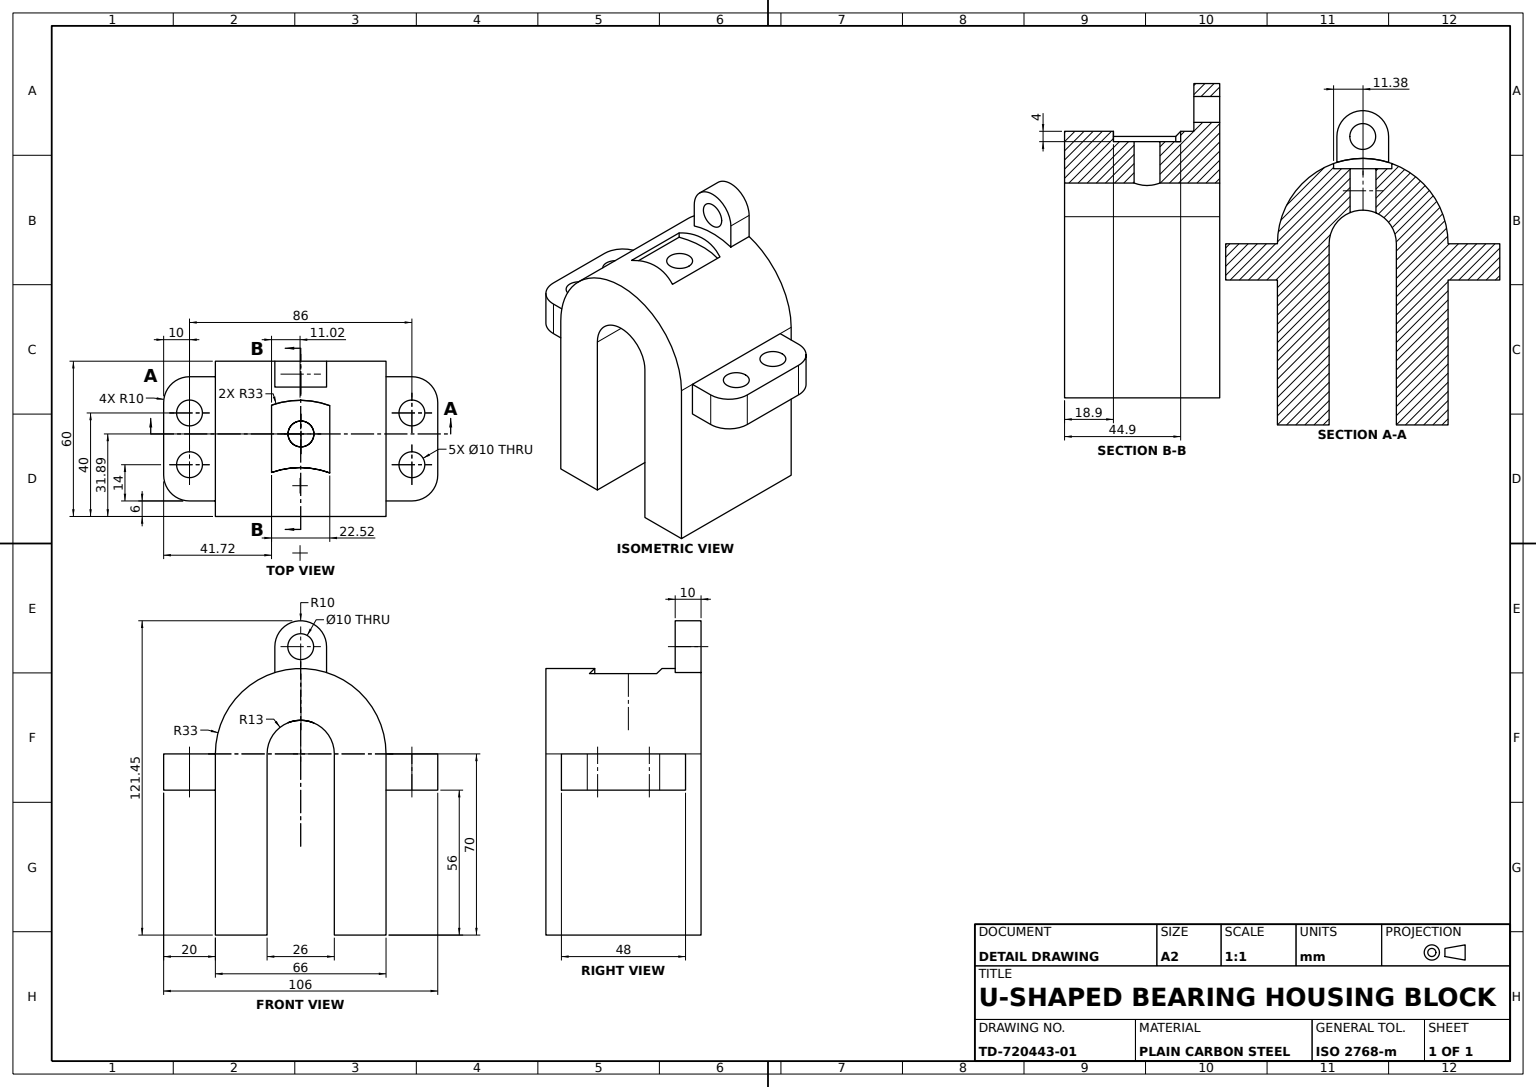
from build123d import *

# Parameters (mm, degrees)
HOUSING_BODY_60_DEPTH        = 60
LIFTING_START                = -10
LIFTING_LUG_SKETCH_R         = 5
LIFTING_LUG_DEPTH            = 10
MOUNTING_FLANGES_SKETCH_W    = 20
MOUNTING_FLANGES_SKETCH_H    = 48
MOUNTING_FLANGES_SKETCH_R    = 5
MOUNTING_FLANGES_14_DEPTH    = 14
FLANGE_CORNER_FILLET_R10_A_R = 10
FLANGE_CORNER_FILLET_R10_B_R = 10
FLANGE_CORNER_FILLET_R10_C_R = 10
FLANGE_CORNER_FILLET_R10_D_R = 10
TOP_RECESS_4_DEEP_DEPTH      = 4
RECESS_HOLE_SKETCH_R         = 5
RECESS_HOLE_DEPTH            = 145.211650056


with BuildPart() as part:
    # Body Profile Sketch → Housing Body 60 (new body)
    with BuildSketch(Plane.XY):
        with BuildLine():
            Line((0, 0), (0, 70))
            ThreePointArc((0, 70), (33, 103), (66, 70))
            Line((66, 70), (66, 0))
            Line((66, 0), (46, 0))
            Line((46, 0), (46, 70))
            ThreePointArc((46, 70), (33, 83), (20, 70))
            Line((20, 70), (20, 0))
            Line((20, 0), (0, 0))
        make_face()
    extrude(amount=-HOUSING_BODY_60_DEPTH)

    # Lifting Lug Sketch → Lifting Lug (add)
    with BuildSketch(Plane(origin=(0, 0, -60), x_dir=(-1, 0, 0), z_dir=(0, 0, -1)).offset(LIFTING_START)):
        with BuildLine():
            Line((-43, 101.448370387), (-43, 111.448370387))
            ThreePointArc((-43, 111.448370387), (-33, 121.448370387), (-23, 111.448370387))
            Line((-23, 111.448370387), (-23, 101.448370387))
            ThreePointArc((-23, 101.448370387), (-33, 103), (-43, 101.448370387))
        make_face()
        with Locations((-33, 111.448370387)):
            Circle(LIFTING_LUG_SKETCH_R, mode=Mode.SUBTRACT)
    extrude(amount=LIFTING_LUG_DEPTH)

    # Mounting Flanges Sketch → Mounting Flanges 14 (add)
    # profile 1 of 2: a face of its own
    with BuildSketch(Plane(origin=(0, 70, 0), x_dir=(1, 0, 0), z_dir=(0, 1, 0))):
        with Locations((76, 30)):
            Rectangle(MOUNTING_FLANGES_SKETCH_W, MOUNTING_FLANGES_SKETCH_H)
        with Locations(Location((76, 20, 0), (0, 0, 270))):
            Circle(MOUNTING_FLANGES_SKETCH_R, mode=Mode.SUBTRACT)
        with Locations(Location((76, 40, 0), (0, 0, 270))):
            Circle(MOUNTING_FLANGES_SKETCH_R, mode=Mode.SUBTRACT)
    # profile 2 of 2: a face of its own
    with BuildSketch(Plane(origin=(0, 70, 0), x_dir=(1, 0, 0), z_dir=(0, 1, 0))):
        with Locations((-10, 30)):
            Rectangle(MOUNTING_FLANGES_SKETCH_W, MOUNTING_FLANGES_SKETCH_H)
        with Locations(Location((-10, 40, 0), (0, 0, 90))):
            Circle(MOUNTING_FLANGES_SKETCH_R, mode=Mode.SUBTRACT)
        with Locations(Location((-10, 20, 0), (0, 0, 90))):
            Circle(MOUNTING_FLANGES_SKETCH_R, mode=Mode.SUBTRACT)
    extrude(amount=-MOUNTING_FLANGES_14_DEPTH)

    # Flange Corner Fillet R10 A
    flange_corner_fillet_r10_a_edges = [part.edges().sort_by_distance(p)[0] for p in [
        (86, 63, -54),
    ]]
    fillet(flange_corner_fillet_r10_a_edges, radius=FLANGE_CORNER_FILLET_R10_A_R)

    # Flange Corner Fillet R10 B
    flange_corner_fillet_r10_b_edges = [part.edges().sort_by_distance(p)[0] for p in [
        (86, 63, -6),
    ]]
    fillet(flange_corner_fillet_r10_b_edges, radius=FLANGE_CORNER_FILLET_R10_B_R)

    # Flange Corner Fillet R10 C
    flange_corner_fillet_r10_c_edges = [part.edges().sort_by_distance(p)[0] for p in [
        (-20, 63, -54),
    ]]
    fillet(flange_corner_fillet_r10_c_edges, radius=FLANGE_CORNER_FILLET_R10_C_R)

    # Flange Corner Fillet R10 D
    flange_corner_fillet_r10_d_edges = [part.edges().sort_by_distance(p)[0] for p in [
        (-20, 63, -6),
    ]]
    fillet(flange_corner_fillet_r10_d_edges, radius=FLANGE_CORNER_FILLET_R10_D_R)

    # Top Recess Sketch → Top Recess 4 Deep (cut)
    with BuildSketch(Plane(origin=(0, 103, 0), x_dir=(1, 0, 0), z_dir=(0, 1, 0))):
        with BuildLine():
            Line((21.724814581, 43), (21.724814581, 17))
            ThreePointArc((21.724814581, 17), (33, 18.894718879), (44.244993393, 16.828347794))
            Line((44.244993393, 16.828347794), (44.244993393, 42.828347794))
            ThreePointArc((44.244993393, 42.828347794), (33, 44.894718879), (21.724814581, 43))
        make_face()
    extrude(amount=-TOP_RECESS_4_DEEP_DEPTH, mode=Mode.SUBTRACT)

    # Recess Hole Sketch → Recess Hole (cut, through all)
    with BuildSketch(Plane(origin=(0, 99, 0), x_dir=(1, 0, 0), z_dir=(0, 1, 0))):
        with Locations(Location((33.108870808, 31.892430073, 0), (0, 0, 180))):
            Circle(RECESS_HOLE_SKETCH_R)
    extrude(amount=-RECESS_HOLE_DEPTH, mode=Mode.SUBTRACT)


solid = part.part
